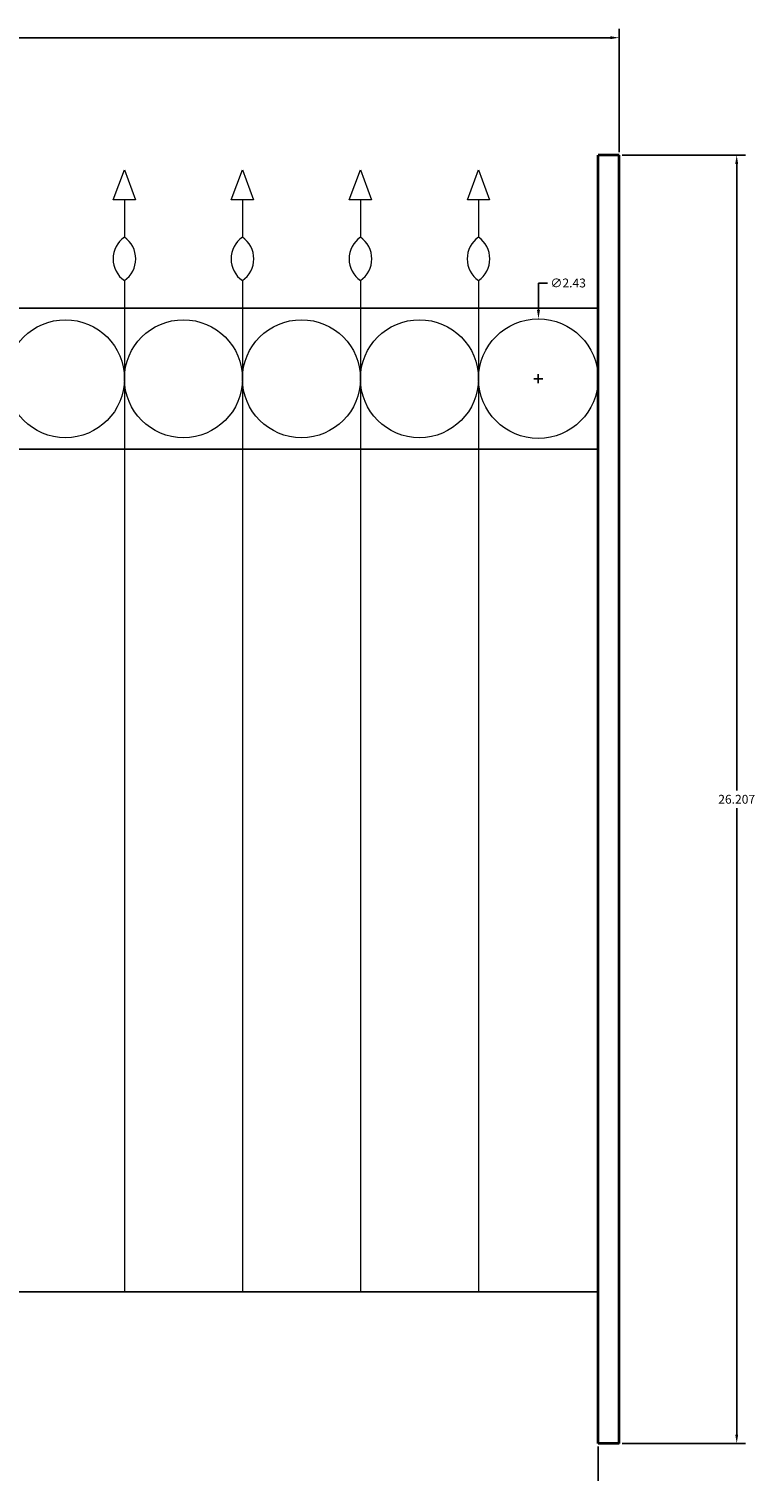
# Model space of a CAD drawing. Units: inches. Extents: x 756 to 915, y 488 to 695.
# Tile 6 of 25: x 844 to 859, y 512 to 541. Entities that reach past the tile are written whole.
import ezdxf

# ---------------------------------------------------------------- set-up
doc = ezdxf.new("R2010")
doc.units = ezdxf.units.IN
doc.header["$MEASUREMENT"] = 0
for name, color, linetype, lineweight in [('L-FENC-PCKT', 7, 'Continuous', 18), ('L-FENC-POST', 7, 'Continuous', 35), ('L-FENC-RAIL', 7, 'Continuous', 25), ('L-FENC-RING', 7, 'Continuous', 18), ('M-DIMS', 2, 'Continuous', 18)]:
    doc.layers.add(name, color=color, linetype=linetype, lineweight=lineweight)
doc.styles.get("Standard").update_dxf_attribs({"font": 'arial.ttf'})
doc.dimstyles.get("Standard").update_dxf_attribs({"dimtxt": 0.18, "dimasz": 0.18, "dimexe": 0.18, "dimexo": 0.0625, "dimgap": 0.09, "dimtad": 0, "dimtih": 1, "dimtoh": 1, "dimdec": 0, "dimzin": 0, "dimdsep": 46, "dimlunit": 3, "dimtxsty": 'Standard', "dimcen": 0.09, "dimadec": 0, "dimazin": 0, "dimtfac": 1, "dimtdec": 0, "dimtofl": 0, "dimtmove": 0, "dimatfit": 3, "dimfxl": 1, "dimtolj": 1, "dimtzin": 0, "dimarcsym": 0})

# ---------------------------------------------------------------- blocks, each defined once
blk = doc.blocks.new('PICKET-MAJESTIC-FLUSH')
for p, q in [((0.231, 22.214), (0.231, 21.456)), ((0.231, 20.573), (0.231, 0))]:
    blk.add_line(p, q)
blk.add_lwpolyline([(0.231, 22.214), (0.004, 22.214), (0.231, 22.826), (0.458, 22.214)], close=True)
blk.add_lwpolyline([(0.231, 20.573, 0.522719), (0.231, 21.456, 0.522719)], format="xyb", close=True)
blk = doc.blocks.new('FENCE-POST-RIGHT')
for p, q in [((0, 26.207), (0, 0)), ((0, 26.207), (0.427, 26.207)), ((0.427, 26.207), (0.427, 0)), ((0, 0), (0.427, 0))]:
    blk.add_line(p, q)
blk = doc.blocks.new('FENCE-PLUS-RING-BAND')
for centre, radius in [((1.286, 1.286), 1.286), ((3.773, 1.286), 1.2), ((6.173, 1.286), 1.2), ((8.572, 1.286), 1.2), ((10.972, 1.286), 1.2), ((13.372, 1.286), 1.2), ((15.772, 1.286), 1.2), ((18.172, 1.286), 1.2), ((20.572, 1.286), 1.2), ((22.972, 1.286), 1.2), ((25.372, 1.286), 1.2), ((27.772, 1.286), 1.2), ((30.172, 1.286), 1.2), ((32.572, 1.286), 1.2), ((34.971, 1.286), 1.2), ((37.388, 1.286), 1.217)]:
    blk.add_circle(centre, radius)
blk = doc.blocks.new('*D76')
at = {"layer": 'Defpoints', "color": 0, "transparency": 16777216}
for p in [(856.101, 541.142), (816.643, 538.752), (856.101, 538.752)]:
    blk.add_point(p, dxfattribs=at)
at = {"layer": 'M-DIMS', "color": 0, "lineweight": -2, "transparency": 16777216}
for p, q in [((816.643, 538.814), (816.643, 541.322)), ((816.823, 541.142), (835.978, 541.142)), ((855.921, 541.142), (836.765, 541.142)), ((856.101, 538.814), (856.101, 541.322))]:
    blk.add_line(p, q, dxfattribs=at)
at = {"layer": 'M-DIMS', "color": 0, "transparency": 16777216}
for points in [[(816.823, 541.172), (816.823, 541.112), (816.643, 541.142)], [(855.921, 541.172), (855.921, 541.112), (856.101, 541.142)]]:
    blk.add_solid(points, dxfattribs=at)
at = {"layer": 'M-DIMS', "color": 0, "transparency": 16777216, "insert": (836.372, 541.142), "char_height": 0.18, "attachment_point": 5}
blk.add_mtext('\\A1;39.46', dxfattribs=at)
blk = doc.blocks.new('*D77')
at = {"layer": 'Defpoints', "color": 0, "transparency": 16777216}
for p in [(856.101, 538.752), (858.491, 538.752), (856.101, 512.545)]:
    blk.add_point(p, dxfattribs=at)
at = {"layer": 'M-DIMS', "color": 0, "lineweight": -2, "transparency": 16777216}
for p, q in [((856.163, 538.752), (858.671, 538.752)), ((858.491, 538.572), (858.491, 525.83)), ((858.491, 512.725), (858.491, 525.466)), ((856.163, 512.545), (858.671, 512.545))]:
    blk.add_line(p, q, dxfattribs=at)
at = {"layer": 'M-DIMS', "color": 0, "transparency": 16777216}
for points in [[(858.461, 538.572), (858.521, 538.572), (858.491, 538.752)], [(858.461, 512.725), (858.521, 512.725), (858.491, 512.545)]]:
    blk.add_solid(points, dxfattribs=at)
at = {"layer": 'M-DIMS', "color": 0, "transparency": 16777216, "insert": (858.491, 525.648), "char_height": 0.18, "attachment_point": 5}
blk.add_mtext('\\A1;26.207', dxfattribs=at)
blk = doc.blocks.new('*D78')
at = {"layer": 'Defpoints', "color": 0, "transparency": 16777216}
for p in [(817.069, 512.545), (855.674, 512.545), (855.674, 510.155)]:
    blk.add_point(p, dxfattribs=at)
at = {"layer": 'M-DIMS', "color": 0, "lineweight": -2, "transparency": 16777216}
for p, q in [((817.069, 512.482), (817.069, 509.975)), ((855.674, 512.482), (855.674, 509.975)), ((817.249, 510.155), (835.908, 510.155)), ((855.494, 510.155), (836.836, 510.155))]:
    blk.add_line(p, q, dxfattribs=at)
at = {"layer": 'M-DIMS', "color": 0, "transparency": 16777216}
for points in [[(817.249, 510.185), (817.249, 510.125), (817.069, 510.155)], [(855.494, 510.185), (855.494, 510.125), (855.674, 510.155)]]:
    blk.add_solid(points, dxfattribs=at)
at = {"layer": 'M-DIMS', "color": 0, "transparency": 16777216, "insert": (836.372, 510.155), "char_height": 0.18, "attachment_point": 5}
blk.add_mtext('\\A1;38.605', dxfattribs=at)
blk = doc.blocks.new('*D89')
at = {"layer": 'Defpoints', "color": 0, "transparency": 16777216}
for p in [(854.46, 535.421), (854.455, 532.988)]:
    blk.add_point(p, dxfattribs=at)
at = {"layer": 'M-DIMS', "color": 0, "lineweight": -2, "transparency": 16777216}
for p, q in [((854.462, 536.151), (854.46, 535.601)), ((854.642, 536.151), (854.462, 536.151)), ((854.367, 534.204), (854.547, 534.204)), ((854.457, 534.114), (854.457, 534.294))]:
    blk.add_line(p, q, dxfattribs=at)
at = {"layer": 'M-DIMS', "color": 0, "transparency": 16777216}
blk.add_solid([(854.43, 535.601), (854.49, 535.601), (854.46, 535.421)], dxfattribs=at)
at = {"layer": 'M-DIMS', "color": 0, "transparency": 16777216, "insert": (855.063, 536.151), "char_height": 0.18, "attachment_point": 5}
blk.add_mtext('\\A1;∅2.43', dxfattribs=at)

msp = doc.modelspace()

# ---------------------------------------------------------------- linework, layer by layer
at = {"layer": 'L-FENC-RAIL'}
for p, q in [((817.0694, 535.6365), (855.6743, 535.6365)), ((817.0694, 532.7722), (855.6743, 532.7722)), ((817.0694, 515.6263), (855.6743, 515.6263))]:
    msp.add_line(p, q, dxfattribs=at)

# ---------------------------------------------------------------- block references
at = {"layer": 'L-FENC-PCKT'}
for p in [(845.81, 515.6267), (848.2099, 515.6267), (850.6098, 515.6267), (853.0098, 515.6267)]:
    msp.add_blockref('PICKET-MAJESTIC-FLUSH', p, dxfattribs=at)
at = {"layer": 'L-FENC-POST', "rotation": 180}
msp.add_blockref('FENCE-POST-RIGHT', (856.1011, 538.7516), dxfattribs=at)
at = {"layer": 'L-FENC-RING'}
msp.add_blockref('FENCE-PLUS-RING-BAND', (817.0693, 532.9183), dxfattribs=at)

# ---------------------------------------------------------------- dimensions: what is measured, and where the dimension line sits
at = {"layer": 'M-DIMS'}
for base, p1, p2, override, picture, middle in [((856.1009, 541.1415), (816.6428, 538.7515), (856.1009, 538.7515), {"dimdec": 2, "dimlfac": 1, "dimrnd": 0, "dimzin": 0, "dimdsep": 46, "dimlunit": 2}, '*D76', (836.3719, 541.1415)), ((855.6743, 510.1547), (817.0694, 512.5447), (855.6743, 512.5447), {"dimdec": 3, "dimlfac": 1, "dimrnd": 0, "dimzin": 0, "dimdsep": 46, "dimlunit": 2}, '*D78', (836.3719, 510.1547))]:
    dim = msp.add_linear_dim(base=base, p1=p1, p2=p2, dimstyle='Standard', override=override, dxfattribs=at)
    dim.commit()
    dim.dimension.update_dxf_attribs({"geometry": picture, "text_midpoint": middle})
dim = msp.add_linear_dim(base=(858.4909, 538.7515), p1=(856.1009, 512.5447), p2=(856.1009, 538.7515), angle=90, dimstyle='Standard', override={"dimdec": 3, "dimlfac": 1, "dimrnd": 0, "dimzin": 0, "dimdsep": 46, "dimlunit": 2}, dxfattribs=at)
dim.commit()
dim.dimension.update_dxf_attribs({"geometry": '*D77', "text_midpoint": (858.4909, 525.6481)})
dim = msp.add_diameter_dim_2p(p1=(854.4549, 532.9875), p2=(854.46, 535.4211), dimstyle='Standard', override={"dimdec": 2, "dimlfac": 1, "dimrnd": 0, "dimzin": 0, "dimdsep": 46, "dimlunit": 2}, dxfattribs=at)
dim.commit()
dim.dimension.update_dxf_attribs({"geometry": '*D89', "text_midpoint": (855.0632, 536.1512), "dimtype": 163})

doc.saveas('drawing.dxf')
